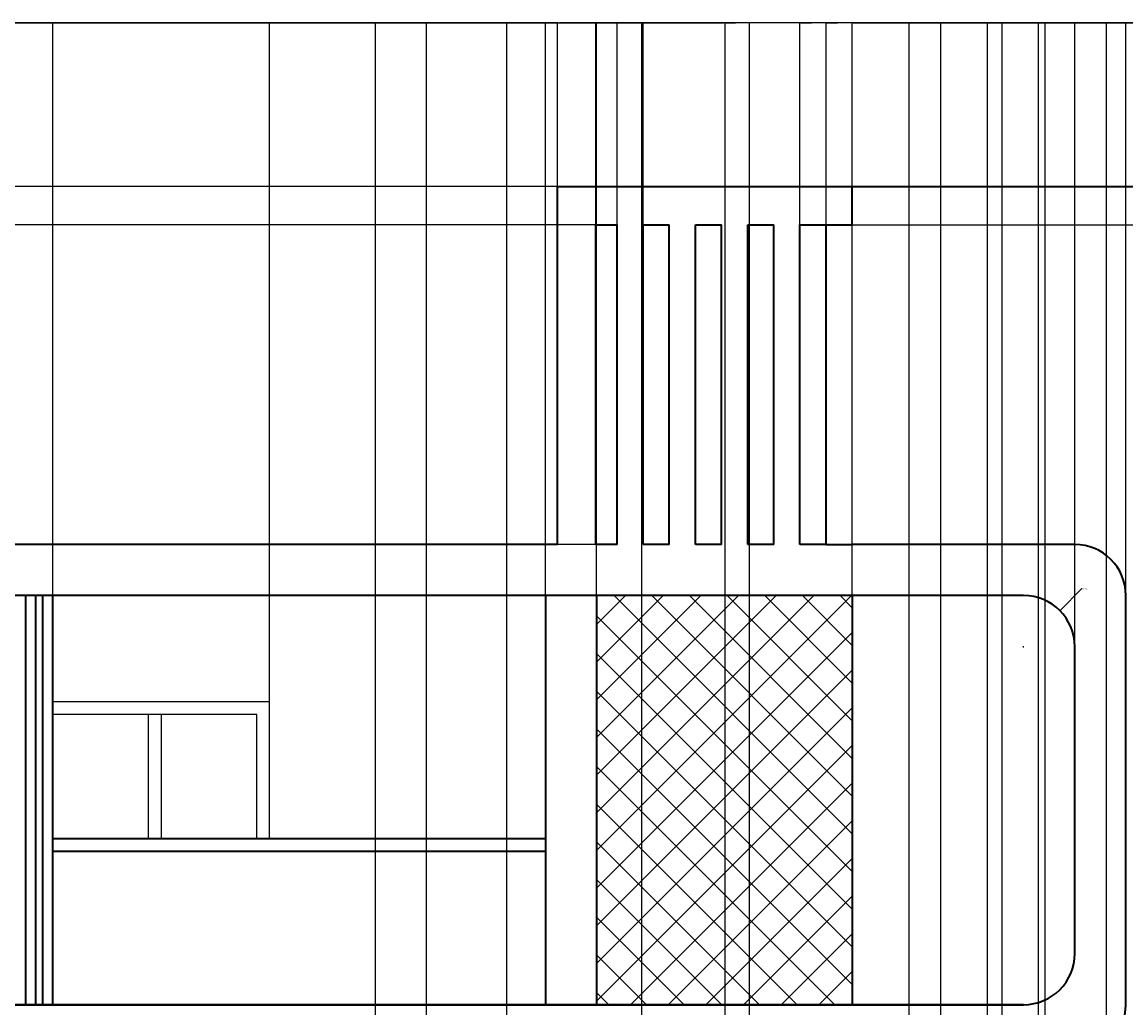
# Model space of a CAD drawing. Units: inches. Extents: x -15 to 605, y -220 to 570.
# Tile 9 of 10: x 138 to 397, y 339 to 570. Entities that reach past the tile are written whole.
import ezdxf

# ---------------------------------------------------------------- set-up
doc = ezdxf.new("R2010")
doc.units = ezdxf.units.IN
doc.header["$MEASUREMENT"] = 0
for name, color, linetype, lineweight in [('A-ANNO-DIMS', 2, 'Continuous', 18), ('A-ELEV', 7, 'Continuous', 35), ('A-ELEV-PATT', 8, 'Continuous', 13), ('A-GLAZ', 4, 'Continuous', 25)]:
    doc.layers.add(name, color=color, linetype=linetype, lineweight=lineweight)
doc.styles.get("Standard").update_dxf_attribs({"font": 'arial.ttf'})
doc.dimstyles.get("Standard").update_dxf_attribs({"dimtxt": 0.18, "dimasz": 0.18, "dimexe": 0.18, "dimexo": 0.0625, "dimgap": 0.09, "dimtad": 0, "dimtih": 1, "dimtoh": 1, "dimdec": 4, "dimzin": 0, "dimdsep": 46, "dimtxsty": 'Standard', "dimcen": 0.09, "dimadec": 0, "dimazin": 0, "dimtfac": 1, "dimtdec": 4, "dimtofl": 0, "dimtmove": 0, "dimatfit": 3, "dimfxl": 1, "dimtolj": 1, "dimtzin": 0, "dimarcsym": 0})

# ---------------------------------------------------------------- blocks, each defined once
blk = doc.blocks.new('WIN-ELEV')
for p, q in [((22.41, 29.07), (22.41, 0)), ((25.41, 29.07), (25.41, 0))]:
    blk.add_line(p, q)
for points in [[(50.87, 0), (50.87, 32.07), (0, 32.07)], [(47.87, 0), (47.87, 29.07), (0, 29.07)]]:
    blk.add_lwpolyline(points)
blk = doc.blocks.new('*D8')
at = {"layer": 'A-ANNO-DIMS', "color": 0, "lineweight": -2, "transparency": 16777216}
for p, q in [((23.99, 3.88), (23.99, 570.4)), ((24.17, 570.22), (263.7, 570.22)), ((503.81, 570.22), (264.28, 570.22)), ((503.99, 531.88), (503.99, 570.4))]:
    blk.add_line(p, q, dxfattribs=at)
at = {"layer": 'A-ANNO-DIMS', "color": 0, "transparency": 16777216}
for points in [[(24.17, 570.25), (24.17, 570.19), (23.99, 570.22)], [(503.81, 570.25), (503.81, 570.19), (503.99, 570.22)]]:
    blk.add_solid(points, dxfattribs=at)
at = {"layer": 'Defpoints', "color": 0, "transparency": 16777216}
for p in [(503.99, 570.22), (503.99, 531.82), (23.99, 3.82)]:
    blk.add_point(p, dxfattribs=at)
at = {"layer": 'A-ANNO-DIMS', "color": 0, "transparency": 16777216, "insert": (263.99, 570.22), "char_height": 0.18, "attachment_point": 5}
blk.add_mtext('\\A1;480', dxfattribs=at)
blk = doc.blocks.new('*D9')
at = {"layer": 'A-ANNO-DIMS', "color": 0, "lineweight": -2, "transparency": 16777216}
for p, q in [((503.92, 531.82), (-14.59, 531.82)), ((-14.41, 531.64), (-14.41, 208)), ((-14.41, -116), (-14.41, 207.64)), ((23.92, -116.18), (-14.59, -116.18))]:
    blk.add_line(p, q, dxfattribs=at)
at = {"layer": 'A-ANNO-DIMS', "color": 0, "transparency": 16777216}
for points in [[(-14.44, 531.64), (-14.38, 531.64), (-14.41, 531.82)], [(-14.44, -116), (-14.38, -116), (-14.41, -116.18)]]:
    blk.add_solid(points, dxfattribs=at)
at = {"layer": 'Defpoints', "color": 0, "transparency": 16777216}
for p in [(-14.41, 531.82), (503.99, 531.82), (23.99, -116.18)]:
    blk.add_point(p, dxfattribs=at)
at = {"layer": 'A-ANNO-DIMS', "color": 0, "transparency": 16777216, "insert": (-14.41, 207.82), "char_height": 0.18, "attachment_point": 5}
blk.add_mtext('\\A1;648', dxfattribs=at)
blk = doc.blocks.new('*D18')
at = {"layer": 'A-ANNO-DIMS', "color": 0, "lineweight": -2, "transparency": 16777216}
for p, q in [((23.99, 3.88), (23.99, 570.4)), ((24.17, 570.22), (143.44, 570.22)), ((263.64, 570.22), (144.37, 570.22)), ((263.82, 447.88), (263.82, 570.4))]:
    blk.add_line(p, q, dxfattribs=at)
at = {"layer": 'A-ANNO-DIMS', "color": 0, "transparency": 16777216}
for points in [[(24.17, 570.25), (24.17, 570.19), (23.99, 570.22)], [(263.64, 570.25), (263.64, 570.19), (263.82, 570.22)]]:
    blk.add_solid(points, dxfattribs=at)
at = {"layer": 'Defpoints', "color": 0, "transparency": 16777216}
for p in [(263.82, 570.22), (263.82, 447.82), (23.99, 3.82)]:
    blk.add_point(p, dxfattribs=at)
at = {"layer": 'A-ANNO-DIMS', "color": 0, "transparency": 16777216, "insert": (143.9, 570.22), "char_height": 0.18, "attachment_point": 5}
blk.add_mtext('\\A1;239.83', dxfattribs=at)
blk = doc.blocks.new('*D19')
at = {"layer": 'A-ANNO-DIMS', "color": 0, "lineweight": -2, "transparency": 16777216}
for p, q in [((263.82, 531.88), (263.82, 570.4)), ((264, 570.22), (298.01, 570.22)), ((332.81, 570.22), (298.8, 570.22)), ((332.99, 435.88), (332.99, 570.4))]:
    blk.add_line(p, q, dxfattribs=at)
at = {"layer": 'A-ANNO-DIMS', "color": 0, "transparency": 16777216}
for points in [[(264, 570.25), (264, 570.19), (263.82, 570.22)], [(332.81, 570.25), (332.81, 570.19), (332.99, 570.22)]]:
    blk.add_solid(points, dxfattribs=at)
at = {"layer": 'Defpoints', "color": 0, "transparency": 16777216}
for p in [(332.99, 570.22), (263.82, 531.82), (332.99, 435.82)]:
    blk.add_point(p, dxfattribs=at)
at = {"layer": 'A-ANNO-DIMS', "color": 0, "transparency": 16777216, "insert": (298.4, 570.22), "char_height": 0.18, "attachment_point": 5}
blk.add_mtext('\\A1;69.17', dxfattribs=at)
blk = doc.blocks.new('*D20')
at = {"layer": 'A-ANNO-DIMS', "color": 0, "lineweight": -2, "transparency": 16777216}
for p, q in [((332.99, 435.88), (332.99, 570.4)), ((333.17, 570.22), (418.22, 570.22)), ((503.81, 570.22), (418.75, 570.22)), ((503.99, 531.88), (503.99, 570.4))]:
    blk.add_line(p, q, dxfattribs=at)
at = {"layer": 'A-ANNO-DIMS', "color": 0, "transparency": 16777216}
for points in [[(333.17, 570.25), (333.17, 570.19), (332.99, 570.22)], [(503.81, 570.25), (503.81, 570.19), (503.99, 570.22)]]:
    blk.add_solid(points, dxfattribs=at)
at = {"layer": 'Defpoints', "color": 0, "transparency": 16777216}
for p in [(503.99, 570.22), (503.99, 531.82), (332.99, 435.82)]:
    blk.add_point(p, dxfattribs=at)
at = {"layer": 'A-ANNO-DIMS', "color": 0, "transparency": 16777216, "insert": (418.49, 570.22), "char_height": 0.18, "attachment_point": 5}
blk.add_mtext('\\A1;171', dxfattribs=at)
blk = doc.blocks.new('*D54')
at = {"layer": 'A-ANNO-DIMS', "color": 0, "lineweight": -2, "transparency": 16777216}
for p, q in [((63.91, -32.12), (63.91, 570.4)), ((64.09, 570.22), (142.07, 570.22)), ((220.96, 570.22), (142.98, 570.22)), ((221.14, -31.58), (221.14, 570.4))]:
    blk.add_line(p, q, dxfattribs=at)
at = {"layer": 'A-ANNO-DIMS', "color": 0, "transparency": 16777216}
for points in [[(64.09, 570.25), (64.09, 570.19), (63.91, 570.22)], [(220.96, 570.25), (220.96, 570.19), (221.14, 570.22)]]:
    blk.add_solid(points, dxfattribs=at)
at = {"layer": 'Defpoints', "color": 0, "transparency": 16777216}
for p in [(221.14, 570.22), (63.91, -32.18), (221.14, -31.64)]:
    blk.add_point(p, dxfattribs=at)
at = {"layer": 'A-ANNO-DIMS', "color": 0, "transparency": 16777216, "insert": (142.53, 570.22), "char_height": 0.18, "attachment_point": 5}
blk.add_mtext('\\A1;157.24', dxfattribs=at)
blk = doc.blocks.new('*D55')
at = {"layer": 'A-ANNO-DIMS', "color": 0, "lineweight": -2, "transparency": 16777216}
for p, q in [((221.14, -31.58), (221.14, 570.4)), ((221.32, 570.22), (226.93, 570.22)), ((232.96, 570.22), (227.35, 570.22)), ((233.14, -31.58), (233.14, 570.4))]:
    blk.add_line(p, q, dxfattribs=at)
at = {"layer": 'A-ANNO-DIMS', "color": 0, "transparency": 16777216}
for points in [[(221.32, 570.25), (221.32, 570.19), (221.14, 570.22)], [(232.96, 570.25), (232.96, 570.19), (233.14, 570.22)]]:
    blk.add_solid(points, dxfattribs=at)
at = {"layer": 'Defpoints', "color": 0, "transparency": 16777216}
for p in [(233.14, 570.22), (221.14, -31.64), (233.14, -31.64)]:
    blk.add_point(p, dxfattribs=at)
at = {"layer": 'A-ANNO-DIMS', "color": 0, "transparency": 16777216, "insert": (227.14, 570.22), "char_height": 0.18, "attachment_point": 5}
blk.add_mtext('\\A1;12', dxfattribs=at)
blk = doc.blocks.new('*D56')
at = {"layer": 'A-ANNO-DIMS', "color": 0, "lineweight": -2, "transparency": 16777216}
for p, q in [((233.14, -31.58), (233.14, 570.4)), ((233.32, 570.22), (298.47, 570.22)), ((364.53, 570.22), (299.38, 570.22)), ((364.71, -56.12), (364.71, 570.4))]:
    blk.add_line(p, q, dxfattribs=at)
at = {"layer": 'A-ANNO-DIMS', "color": 0, "transparency": 16777216}
for points in [[(233.32, 570.25), (233.32, 570.19), (233.14, 570.22)], [(364.53, 570.25), (364.53, 570.19), (364.71, 570.22)]]:
    blk.add_solid(points, dxfattribs=at)
at = {"layer": 'Defpoints', "color": 0, "transparency": 16777216}
for p in [(364.71, 570.22), (233.14, -31.64), (364.71, -56.18)]:
    blk.add_point(p, dxfattribs=at)
at = {"layer": 'A-ANNO-DIMS', "color": 0, "transparency": 16777216, "insert": (298.93, 570.22), "char_height": 0.18, "attachment_point": 5}
blk.add_mtext('\\A1;131.56', dxfattribs=at)
blk = doc.blocks.new('*D57')
at = {"layer": 'A-ANNO-DIMS', "color": 0, "lineweight": -2, "transparency": 16777216}
for p, q in [((364.71, -56.12), (364.71, 570.4)), ((364.89, 570.22), (370.5, 570.22)), ((376.53, 570.22), (370.92, 570.22)), ((376.71, -44.82), (376.71, 570.4))]:
    blk.add_line(p, q, dxfattribs=at)
at = {"layer": 'A-ANNO-DIMS', "color": 0, "transparency": 16777216}
for points in [[(364.89, 570.25), (364.89, 570.19), (364.71, 570.22)], [(376.53, 570.25), (376.53, 570.19), (376.71, 570.22)]]:
    blk.add_solid(points, dxfattribs=at)
at = {"layer": 'Defpoints', "color": 0, "transparency": 16777216}
for p in [(376.71, 570.22), (376.71, -44.88), (364.71, -56.18)]:
    blk.add_point(p, dxfattribs=at)
at = {"layer": 'A-ANNO-DIMS', "color": 0, "transparency": 16777216, "insert": (370.71, 570.22), "char_height": 0.18, "attachment_point": 5}
blk.add_mtext('\\A1;12', dxfattribs=at)
blk = doc.blocks.new('*D58')
at = {"layer": 'A-ANNO-DIMS', "color": 0, "lineweight": -2, "transparency": 16777216}
for p, q in [((376.71, -44.82), (376.71, 570.4)), ((376.89, 570.22), (419.58, 570.22)), ((462.92, 570.22), (420.23, 570.22)), ((463.1, -45.87), (463.1, 570.4))]:
    blk.add_line(p, q, dxfattribs=at)
at = {"layer": 'A-ANNO-DIMS', "color": 0, "transparency": 16777216}
for points in [[(376.89, 570.25), (376.89, 570.19), (376.71, 570.22)], [(462.92, 570.25), (462.92, 570.19), (463.1, 570.22)]]:
    blk.add_solid(points, dxfattribs=at)
at = {"layer": 'Defpoints', "color": 0, "transparency": 16777216}
for p in [(463.1, 570.22), (376.71, -44.88), (463.1, -45.94)]:
    blk.add_point(p, dxfattribs=at)
at = {"layer": 'A-ANNO-DIMS', "color": 0, "transparency": 16777216, "insert": (419.9, 570.22), "char_height": 0.18, "attachment_point": 5}
blk.add_mtext('\\A1;86.4', dxfattribs=at)
blk = doc.blocks.new('*D60')
at = {"layer": 'A-ANNO-DIMS', "color": 0, "lineweight": -2, "transparency": 16777216}
for p, q in [((346.37, -116.12), (346.37, 570.4)), ((346.55, 570.22), (349.67, 570.22)), ((353.57, 570.22), (350.45, 570.22)), ((353.75, -39.82), (353.75, 570.4))]:
    blk.add_line(p, q, dxfattribs=at)
at = {"layer": 'A-ANNO-DIMS', "color": 0, "transparency": 16777216}
for points in [[(346.55, 570.25), (346.55, 570.19), (346.37, 570.22)], [(353.57, 570.25), (353.57, 570.19), (353.75, 570.22)]]:
    blk.add_solid(points, dxfattribs=at)
at = {"layer": 'Defpoints', "color": 0, "transparency": 16777216}
for p in [(353.75, 570.22), (353.75, -39.88), (346.37, -116.18)]:
    blk.add_point(p, dxfattribs=at)
at = {"layer": 'A-ANNO-DIMS', "color": 0, "transparency": 16777216, "insert": (350.06, 570.22), "char_height": 0.18, "attachment_point": 5}
blk.add_mtext('\\A1;7.384', dxfattribs=at)
blk = doc.blocks.new('*D61')
at = {"layer": 'A-ANNO-DIMS', "color": 0, "lineweight": -2, "transparency": 16777216}
for p, q in [((353.75, -39.82), (353.75, 570.4)), ((353.93, 570.22), (360.55, 570.22)), ((367.95, 570.22), (361.33, 570.22)), ((368.13, -39.82), (368.13, 570.4))]:
    blk.add_line(p, q, dxfattribs=at)
at = {"layer": 'A-ANNO-DIMS', "color": 0, "transparency": 16777216}
for points in [[(353.93, 570.25), (353.93, 570.19), (353.75, 570.22)], [(367.95, 570.25), (367.95, 570.19), (368.13, 570.22)]]:
    blk.add_solid(points, dxfattribs=at)
at = {"layer": 'Defpoints', "color": 0, "transparency": 16777216}
for p in [(368.13, 570.22), (353.75, -39.88), (368.13, -39.88)]:
    blk.add_point(p, dxfattribs=at)
at = {"layer": 'A-ANNO-DIMS', "color": 0, "transparency": 16777216, "insert": (360.94, 570.22), "char_height": 0.18, "attachment_point": 5}
blk.add_mtext('\\A1;14.38', dxfattribs=at)
blk = doc.blocks.new('*D62')
at = {"layer": 'A-ANNO-DIMS', "color": 0, "lineweight": -2, "transparency": 16777216}
for p, q in [((378.23, -39.82), (378.23, 570.4)), ((378.41, 570.22), (385.04, 570.22)), ((392.43, 570.22), (385.81, 570.22)), ((392.61, -39.82), (392.61, 570.4))]:
    blk.add_line(p, q, dxfattribs=at)
at = {"layer": 'A-ANNO-DIMS', "color": 0, "transparency": 16777216}
for points in [[(378.41, 570.25), (378.41, 570.19), (378.23, 570.22)], [(392.43, 570.25), (392.43, 570.19), (392.61, 570.22)]]:
    blk.add_solid(points, dxfattribs=at)
at = {"layer": 'Defpoints', "color": 0, "transparency": 16777216}
for p in [(392.61, 570.22), (378.23, -39.88), (392.61, -39.88)]:
    blk.add_point(p, dxfattribs=at)
at = {"layer": 'A-ANNO-DIMS', "color": 0, "transparency": 16777216, "insert": (385.42, 570.22), "char_height": 0.18, "attachment_point": 5}
blk.add_mtext('\\A1;14.38', dxfattribs=at)
blk = doc.blocks.new('*D69')
at = {"layer": 'A-ANNO-DIMS', "color": 0, "lineweight": -2, "transparency": 16777216}
for p, q in [((263.82, 531.88), (263.82, 570.4)), ((264, 570.22), (268.17, 570.22)), ((272.64, 570.22), (268.47, 570.22)), ((272.82, 522.88), (272.82, 570.4))]:
    blk.add_line(p, q, dxfattribs=at)
at = {"layer": 'A-ANNO-DIMS', "color": 0, "transparency": 16777216}
for points in [[(264, 570.25), (264, 570.19), (263.82, 570.22)], [(272.64, 570.25), (272.64, 570.19), (272.82, 570.22)]]:
    blk.add_solid(points, dxfattribs=at)
at = {"layer": 'Defpoints', "color": 0, "transparency": 16777216}
for p in [(272.82, 570.22), (263.82, 531.82), (272.82, 522.82)]:
    blk.add_point(p, dxfattribs=at)
at = {"layer": 'A-ANNO-DIMS', "color": 0, "transparency": 16777216, "insert": (268.32, 570.22), "char_height": 0.18, "attachment_point": 5}
blk.add_mtext('\\A1;9', dxfattribs=at)
blk = doc.blocks.new('*D70')
at = {"layer": 'A-ANNO-DIMS', "color": 0, "lineweight": -2, "transparency": 16777216}
for p, q in [((272.82, 522.88), (272.82, 570.4)), ((273, 570.22), (274.91, 570.22)), ((277.62, 570.22), (275.71, 570.22)), ((277.8, 522.88), (277.8, 570.4))]:
    blk.add_line(p, q, dxfattribs=at)
at = {"layer": 'A-ANNO-DIMS', "color": 0, "transparency": 16777216}
for points in [[(273, 570.25), (273, 570.19), (272.82, 570.22)], [(277.62, 570.25), (277.62, 570.19), (277.8, 570.22)]]:
    blk.add_solid(points, dxfattribs=at)
at = {"layer": 'Defpoints', "color": 0, "transparency": 16777216}
for p in [(277.8, 570.22), (272.82, 522.82), (277.8, 522.82)]:
    blk.add_point(p, dxfattribs=at)
at = {"layer": 'A-ANNO-DIMS', "color": 0, "transparency": 16777216, "insert": (275.31, 570.22), "char_height": 0.18, "attachment_point": 5}
blk.add_mtext('\\A1;4.987', dxfattribs=at)
blk = doc.blocks.new('*D71')
at = {"layer": 'A-ANNO-DIMS', "color": 0, "lineweight": -2, "transparency": 16777216}
for p, q in [((277.8, 522.88), (277.8, 570.4)), ((277.98, 570.22), (280.48, 570.22)), ((283.75, 570.22), (281.26, 570.22)), ((283.93, 522.88), (283.93, 570.4))]:
    blk.add_line(p, q, dxfattribs=at)
at = {"layer": 'A-ANNO-DIMS', "color": 0, "transparency": 16777216}
for points in [[(277.98, 570.25), (277.98, 570.19), (277.8, 570.22)], [(283.75, 570.25), (283.75, 570.19), (283.93, 570.22)]]:
    blk.add_solid(points, dxfattribs=at)
at = {"layer": 'Defpoints', "color": 0, "transparency": 16777216}
for p in [(283.93, 570.22), (277.8, 522.82), (283.93, 522.82)]:
    blk.add_point(p, dxfattribs=at)
at = {"layer": 'A-ANNO-DIMS', "color": 0, "transparency": 16777216, "insert": (280.87, 570.22), "char_height": 0.18, "attachment_point": 5}
blk.add_mtext('\\A1;6.132', dxfattribs=at)
blk = doc.blocks.new('*D72')
at = {"layer": 'A-ANNO-DIMS', "color": 0, "lineweight": -2, "transparency": 16777216}
for p, q in [((320.72, 522.88), (320.72, 570.4)), ((320.9, 570.22), (323.4, 570.22)), ((326.68, 570.22), (324.18, 570.22)), ((326.86, 522.88), (326.86, 570.4))]:
    blk.add_line(p, q, dxfattribs=at)
at = {"layer": 'A-ANNO-DIMS', "color": 0, "transparency": 16777216}
for points in [[(320.9, 570.25), (320.9, 570.19), (320.72, 570.22)], [(326.68, 570.25), (326.68, 570.19), (326.86, 570.22)]]:
    blk.add_solid(points, dxfattribs=at)
at = {"layer": 'Defpoints', "color": 0, "transparency": 16777216}
for p in [(326.86, 570.22), (320.72, 522.82), (326.86, 522.82)]:
    blk.add_point(p, dxfattribs=at)
at = {"layer": 'A-ANNO-DIMS', "color": 0, "transparency": 16777216, "insert": (323.79, 570.22), "char_height": 0.18, "attachment_point": 5}
blk.add_mtext('\\A1;6.132', dxfattribs=at)
blk = doc.blocks.new('*D73')
at = {"layer": 'A-ANNO-DIMS', "color": 0, "lineweight": -2, "transparency": 16777216}
for p, q in [((326.86, 522.88), (326.86, 570.4)), ((327.04, 570.22), (329.53, 570.22)), ((332.81, 570.22), (330.31, 570.22)), ((332.99, 522.88), (332.99, 570.4))]:
    blk.add_line(p, q, dxfattribs=at)
at = {"layer": 'A-ANNO-DIMS', "color": 0, "transparency": 16777216}
for points in [[(327.04, 570.25), (327.04, 570.19), (326.86, 570.22)], [(332.81, 570.25), (332.81, 570.19), (332.99, 570.22)]]:
    blk.add_solid(points, dxfattribs=at)
at = {"layer": 'Defpoints', "color": 0, "transparency": 16777216}
for p in [(332.99, 570.22), (326.86, 522.82), (332.99, 522.82)]:
    blk.add_point(p, dxfattribs=at)
at = {"layer": 'A-ANNO-DIMS', "color": 0, "transparency": 16777216, "insert": (329.92, 570.22), "char_height": 0.18, "attachment_point": 5}
blk.add_mtext('\\A1;6.132', dxfattribs=at)
blk = doc.blocks.new('*D74')
at = {"layer": 'A-ANNO-DIMS', "color": 0, "lineweight": -2, "transparency": 16777216}
for p, q in [((272.75, 522.82), (-14.59, 522.82)), ((-14.41, 522.64), (-14.41, 485.5)), ((-14.41, 448), (-14.41, 485.14)), ((272.75, 447.82), (-14.59, 447.82))]:
    blk.add_line(p, q, dxfattribs=at)
at = {"layer": 'A-ANNO-DIMS', "color": 0, "transparency": 16777216}
for points in [[(-14.44, 522.64), (-14.38, 522.64), (-14.41, 522.82)], [(-14.44, 448), (-14.38, 448), (-14.41, 447.82)]]:
    blk.add_solid(points, dxfattribs=at)
at = {"layer": 'Defpoints', "color": 0, "transparency": 16777216}
for p in [(-14.41, 522.82), (272.82, 522.82), (272.82, 447.82)]:
    blk.add_point(p, dxfattribs=at)
at = {"layer": 'A-ANNO-DIMS', "color": 0, "transparency": 16777216, "insert": (-14.41, 485.32), "char_height": 0.18, "attachment_point": 5}
blk.add_mtext('\\A1;75', dxfattribs=at)
blk = doc.blocks.new('*D75')
at = {"layer": 'A-ANNO-DIMS', "color": 0, "lineweight": -2, "transparency": 16777216}
for p, q in [((333.05, 531.82), (605.3, 531.82)), ((605.12, 531.64), (605.12, 527.5)), ((605.12, 523), (605.12, 527.14)), ((333.05, 522.82), (605.3, 522.82))]:
    blk.add_line(p, q, dxfattribs=at)
at = {"layer": 'A-ANNO-DIMS', "color": 0, "transparency": 16777216}
for points in [[(605.09, 531.64), (605.15, 531.64), (605.12, 531.82)], [(605.09, 523), (605.15, 523), (605.12, 522.82)]]:
    blk.add_solid(points, dxfattribs=at)
at = {"layer": 'Defpoints', "color": 0, "transparency": 16777216}
for p in [(332.99, 531.82), (605.12, 531.82), (332.99, 522.82)]:
    blk.add_point(p, dxfattribs=at)
at = {"layer": 'A-ANNO-DIMS', "color": 0, "transparency": 16777216, "insert": (605.12, 527.32), "char_height": 0.18, "attachment_point": 5}
blk.add_mtext('\\A1;9', dxfattribs=at)
blk = doc.blocks.new('*D76')
at = {"layer": 'A-ANNO-DIMS', "color": 0, "lineweight": -2, "transparency": 16777216}
for p, q in [((272.92, 339.82), (-14.59, 339.82)), ((-14.41, 339.64), (-14.41, 334)), ((-14.41, 328), (-14.41, 333.64)), ((272.92, 327.82), (-14.59, 327.82))]:
    blk.add_line(p, q, dxfattribs=at)
at = {"layer": 'A-ANNO-DIMS', "color": 0, "transparency": 16777216}
for points in [[(-14.44, 339.64), (-14.38, 339.64), (-14.41, 339.82)], [(-14.44, 328), (-14.38, 328), (-14.41, 327.82)]]:
    blk.add_solid(points, dxfattribs=at)
at = {"layer": 'Defpoints', "color": 0, "transparency": 16777216}
for p in [(-14.41, 339.82), (272.99, 339.82), (272.99, 327.82)]:
    blk.add_point(p, dxfattribs=at)
at = {"layer": 'A-ANNO-DIMS', "color": 0, "transparency": 16777216, "insert": (-14.41, 333.82), "char_height": 0.18, "attachment_point": 5}
blk.add_mtext('\\A1;12', dxfattribs=at)
blk = doc.blocks.new('*D77')
at = {"layer": 'A-ANNO-DIMS', "color": 0, "lineweight": -2, "transparency": 16777216}
for p, q in [((272.92, 435.82), (-14.59, 435.82)), ((-14.41, 435.64), (-14.41, 388)), ((-14.41, 340), (-14.41, 387.64)), ((272.92, 339.82), (-14.59, 339.82))]:
    blk.add_line(p, q, dxfattribs=at)
at = {"layer": 'A-ANNO-DIMS', "color": 0, "transparency": 16777216}
for points in [[(-14.44, 435.64), (-14.38, 435.64), (-14.41, 435.82)], [(-14.44, 340), (-14.38, 340), (-14.41, 339.82)]]:
    blk.add_solid(points, dxfattribs=at)
at = {"layer": 'Defpoints', "color": 0, "transparency": 16777216}
for p in [(-14.41, 435.82), (272.99, 435.82), (272.99, 339.82)]:
    blk.add_point(p, dxfattribs=at)
at = {"layer": 'A-ANNO-DIMS', "color": 0, "transparency": 16777216, "insert": (-14.41, 387.82), "char_height": 0.18, "attachment_point": 5}
blk.add_mtext('\\A1;96', dxfattribs=at)
blk = doc.blocks.new('*D78')
at = {"layer": 'A-ANNO-DIMS', "color": 0, "lineweight": -2, "transparency": 16777216}
for p, q in [((272.75, 447.82), (-14.59, 447.82)), ((-14.41, 447.64), (-14.41, 442)), ((-14.41, 436), (-14.41, 441.64)), ((272.92, 435.82), (-14.59, 435.82))]:
    blk.add_line(p, q, dxfattribs=at)
at = {"layer": 'A-ANNO-DIMS', "color": 0, "transparency": 16777216}
for points in [[(-14.44, 447.64), (-14.38, 447.64), (-14.41, 447.82)], [(-14.44, 436), (-14.38, 436), (-14.41, 435.82)]]:
    blk.add_solid(points, dxfattribs=at)
at = {"layer": 'Defpoints', "color": 0, "transparency": 16777216}
for p in [(-14.41, 447.82), (272.82, 447.82), (272.99, 435.82)]:
    blk.add_point(p, dxfattribs=at)
at = {"layer": 'A-ANNO-DIMS', "color": 0, "transparency": 16777216, "insert": (-14.41, 441.82), "char_height": 0.18, "attachment_point": 5}
blk.add_mtext('\\A1;12', dxfattribs=at)
blk = doc.blocks.new('*D82')
at = {"layer": 'A-ANNO-DIMS', "color": 0, "lineweight": -2, "transparency": 16777216}
for p, q in [((123.03, 339.88), (123.03, 570.4)), ((123.21, 570.22), (133.9, 570.22)), ((145.25, 570.22), (134.55, 570.22)), ((145.43, 339.88), (145.43, 570.4))]:
    blk.add_line(p, q, dxfattribs=at)
at = {"layer": 'A-ANNO-DIMS', "color": 0, "transparency": 16777216}
for points in [[(123.21, 570.25), (123.21, 570.19), (123.03, 570.22)], [(145.25, 570.25), (145.25, 570.19), (145.43, 570.22)]]:
    blk.add_solid(points, dxfattribs=at)
at = {"layer": 'Defpoints', "color": 0, "transparency": 16777216}
for p in [(145.43, 570.22), (123.03, 339.82), (145.43, 339.82)]:
    blk.add_point(p, dxfattribs=at)
at = {"layer": 'A-ANNO-DIMS', "color": 0, "transparency": 16777216, "insert": (134.23, 570.22), "char_height": 0.18, "attachment_point": 5}
blk.add_mtext('\\A1;22.4', dxfattribs=at)
blk = doc.blocks.new('*D83')
at = {"layer": 'A-ANNO-DIMS', "color": 0, "lineweight": -2, "transparency": 16777216}
for p, q in [((145.43, 339.88), (145.43, 570.4)), ((145.61, 570.22), (170.47, 570.22)), ((196.11, 570.22), (171.25, 570.22)), ((196.29, 378.88), (196.29, 570.4))]:
    blk.add_line(p, q, dxfattribs=at)
at = {"layer": 'A-ANNO-DIMS', "color": 0, "transparency": 16777216}
for points in [[(145.61, 570.25), (145.61, 570.19), (145.43, 570.22)], [(196.11, 570.25), (196.11, 570.19), (196.29, 570.22)]]:
    blk.add_solid(points, dxfattribs=at)
at = {"layer": 'Defpoints', "color": 0, "transparency": 16777216}
for p in [(196.29, 570.22), (196.29, 378.82), (145.43, 339.82)]:
    blk.add_point(p, dxfattribs=at)
at = {"layer": 'A-ANNO-DIMS', "color": 0, "transparency": 16777216, "insert": (170.86, 570.22), "char_height": 0.18, "attachment_point": 5}
blk.add_mtext('\\A1;50.87', dxfattribs=at)
blk = doc.blocks.new('*D84')
at = {"layer": 'A-ANNO-DIMS', "color": 0, "lineweight": -2, "transparency": 16777216}
for p, q in [((196.29, 378.88), (196.29, 570.4)), ((196.47, 570.22), (228.25, 570.22)), ((260.81, 570.22), (229.04, 570.22)), ((260.99, 339.88), (260.99, 570.4))]:
    blk.add_line(p, q, dxfattribs=at)
at = {"layer": 'A-ANNO-DIMS', "color": 0, "transparency": 16777216}
for points in [[(196.47, 570.25), (196.47, 570.19), (196.29, 570.22)], [(260.81, 570.25), (260.81, 570.19), (260.99, 570.22)]]:
    blk.add_solid(points, dxfattribs=at)
at = {"layer": 'Defpoints', "color": 0, "transparency": 16777216}
for p in [(260.99, 570.22), (196.29, 378.82), (260.99, 339.82)]:
    blk.add_point(p, dxfattribs=at)
at = {"layer": 'A-ANNO-DIMS', "color": 0, "transparency": 16777216, "insert": (228.64, 570.22), "char_height": 0.18, "attachment_point": 5}
blk.add_mtext('\\A1;64.69', dxfattribs=at)
blk = doc.blocks.new('*D85')
at = {"layer": 'A-ANNO-DIMS', "color": 0, "lineweight": -2, "transparency": 16777216}
for p, q in [((260.99, 339.88), (260.99, 570.4)), ((261.17, 570.22), (266.78, 570.22)), ((272.81, 570.22), (267.2, 570.22)), ((272.99, 339.88), (272.99, 570.4))]:
    blk.add_line(p, q, dxfattribs=at)
at = {"layer": 'A-ANNO-DIMS', "color": 0, "transparency": 16777216}
for points in [[(261.17, 570.25), (261.17, 570.19), (260.99, 570.22)], [(272.81, 570.25), (272.81, 570.19), (272.99, 570.22)]]:
    blk.add_solid(points, dxfattribs=at)
at = {"layer": 'Defpoints', "color": 0, "transparency": 16777216}
for p in [(272.99, 570.22), (260.99, 339.82), (272.99, 339.82)]:
    blk.add_point(p, dxfattribs=at)
at = {"layer": 'A-ANNO-DIMS', "color": 0, "transparency": 16777216, "insert": (266.99, 570.22), "char_height": 0.18, "attachment_point": 5}
blk.add_mtext('\\A1;12', dxfattribs=at)
blk = doc.blocks.new('*D86')
at = {"layer": 'A-ANNO-DIMS', "color": 0, "lineweight": -2, "transparency": 16777216}
for p, q in [((272.99, 339.88), (272.99, 570.4)), ((273.17, 570.22), (302.77, 570.22)), ((332.81, 570.22), (303.21, 570.22)), ((332.99, 339.88), (332.99, 570.4))]:
    blk.add_line(p, q, dxfattribs=at)
at = {"layer": 'A-ANNO-DIMS', "color": 0, "transparency": 16777216}
for points in [[(273.17, 570.25), (273.17, 570.19), (272.99, 570.22)], [(332.81, 570.25), (332.81, 570.19), (332.99, 570.22)]]:
    blk.add_solid(points, dxfattribs=at)
at = {"layer": 'Defpoints', "color": 0, "transparency": 16777216}
for p in [(332.99, 570.22), (272.99, 339.82), (332.99, 339.82)]:
    blk.add_point(p, dxfattribs=at)
at = {"layer": 'A-ANNO-DIMS', "color": 0, "transparency": 16777216, "insert": (302.99, 570.22), "char_height": 0.18, "attachment_point": 5}
blk.add_mtext('\\A1;60', dxfattribs=at)
blk = doc.blocks.new('*D87')
at = {"layer": 'A-ANNO-DIMS', "color": 0, "lineweight": -2, "transparency": 16777216}
for p, q in [((332.99, 339.88), (332.99, 570.4)), ((333.17, 570.22), (358.77, 570.22)), ((385.01, 570.22), (359.41, 570.22)), ((385.19, 351.88), (385.19, 570.4))]:
    blk.add_line(p, q, dxfattribs=at)
at = {"layer": 'A-ANNO-DIMS', "color": 0, "transparency": 16777216}
for points in [[(333.17, 570.25), (333.17, 570.19), (332.99, 570.22)], [(385.01, 570.25), (385.01, 570.19), (385.19, 570.22)]]:
    blk.add_solid(points, dxfattribs=at)
at = {"layer": 'Defpoints', "color": 0, "transparency": 16777216}
for p in [(385.19, 570.22), (385.19, 351.82), (332.99, 339.82)]:
    blk.add_point(p, dxfattribs=at)
at = {"layer": 'A-ANNO-DIMS', "color": 0, "transparency": 16777216, "insert": (359.09, 570.22), "char_height": 0.18, "attachment_point": 5}
blk.add_mtext('\\A1;52.2', dxfattribs=at)
blk = doc.blocks.new('*D88')
at = {"layer": 'A-ANNO-DIMS', "color": 0, "lineweight": -2, "transparency": 16777216}
for p, q in [((385.19, 351.88), (385.19, 570.4)), ((385.37, 570.22), (390.98, 570.22)), ((397.01, 570.22), (391.4, 570.22)), ((397.19, 339.88), (397.19, 570.4))]:
    blk.add_line(p, q, dxfattribs=at)
at = {"layer": 'A-ANNO-DIMS', "color": 0, "transparency": 16777216}
for points in [[(385.37, 570.25), (385.37, 570.19), (385.19, 570.22)], [(397.01, 570.25), (397.01, 570.19), (397.19, 570.22)]]:
    blk.add_solid(points, dxfattribs=at)
at = {"layer": 'Defpoints', "color": 0, "transparency": 16777216}
for p in [(397.19, 570.22), (385.19, 351.82), (397.19, 339.82)]:
    blk.add_point(p, dxfattribs=at)
at = {"layer": 'A-ANNO-DIMS', "color": 0, "transparency": 16777216, "insert": (391.19, 570.22), "char_height": 0.18, "attachment_point": 5}
blk.add_mtext('\\A1;12', dxfattribs=at)
blk = doc.blocks.new('*D104')
at = {"layer": 'A-ANNO-DIMS', "color": 0, "lineweight": -2, "transparency": 16777216}
for p, q in [((251.99, -56.12), (251.99, 570.4)), ((252.17, 570.22), (267.39, 570.22)), ((283.41, 570.22), (268.18, 570.22)), ((283.59, -84.79), (283.59, 570.4))]:
    blk.add_line(p, q, dxfattribs=at)
at = {"layer": 'A-ANNO-DIMS', "color": 0, "transparency": 16777216}
for points in [[(252.17, 570.25), (252.17, 570.19), (251.99, 570.22)], [(283.41, 570.25), (283.41, 570.19), (283.59, 570.22)]]:
    blk.add_solid(points, dxfattribs=at)
at = {"layer": 'Defpoints', "color": 0, "transparency": 16777216}
for p in [(283.59, 570.22), (251.99, -56.18), (283.59, -84.86)]:
    blk.add_point(p, dxfattribs=at)
at = {"layer": 'A-ANNO-DIMS', "color": 0, "transparency": 16777216, "insert": (267.79, 570.22), "char_height": 0.18, "attachment_point": 5}
blk.add_mtext('\\A1;31.60', dxfattribs=at)
blk = doc.blocks.new('*D105')
at = {"layer": 'A-ANNO-DIMS', "color": 0, "lineweight": -2, "transparency": 16777216}
for p, q in [((283.59, -84.79), (283.59, 570.4)), ((283.77, 570.22), (292.92, 570.22)), ((302.99, 570.22), (293.84, 570.22)), ((303.17, -103.62), (303.17, 570.4))]:
    blk.add_line(p, q, dxfattribs=at)
at = {"layer": 'A-ANNO-DIMS', "color": 0, "transparency": 16777216}
for points in [[(283.77, 570.25), (283.77, 570.19), (283.59, 570.22)], [(302.99, 570.25), (302.99, 570.19), (303.17, 570.22)]]:
    blk.add_solid(points, dxfattribs=at)
at = {"layer": 'Defpoints', "color": 0, "transparency": 16777216}
for p in [(303.17, 570.22), (283.59, -84.86), (303.17, -103.68)]:
    blk.add_point(p, dxfattribs=at)
at = {"layer": 'A-ANNO-DIMS', "color": 0, "transparency": 16777216, "insert": (293.38, 570.22), "char_height": 0.18, "attachment_point": 5}
blk.add_mtext('\\A1;19.585', dxfattribs=at)
blk = doc.blocks.new('*D106')
at = {"layer": 'A-ANNO-DIMS', "color": 0, "lineweight": -2, "transparency": 16777216}
for p, q in [((303.17, -103.62), (303.17, 570.4)), ((303.35, 570.22), (305.62, 570.22)), ((308.68, 570.22), (306.41, 570.22)), ((308.86, -79.16), (308.86, 570.4))]:
    blk.add_line(p, q, dxfattribs=at)
at = {"layer": 'A-ANNO-DIMS', "color": 0, "transparency": 16777216}
for points in [[(303.35, 570.25), (303.35, 570.19), (303.17, 570.22)], [(308.68, 570.25), (308.68, 570.19), (308.86, 570.22)]]:
    blk.add_solid(points, dxfattribs=at)
at = {"layer": 'Defpoints', "color": 0, "transparency": 16777216}
for p in [(308.86, 570.22), (308.86, -79.22), (303.17, -103.68)]:
    blk.add_point(p, dxfattribs=at)
at = {"layer": 'A-ANNO-DIMS', "color": 0, "transparency": 16777216, "insert": (306.02, 570.22), "char_height": 0.18, "attachment_point": 5}
blk.add_mtext('\\A1;5.689', dxfattribs=at)
blk = doc.blocks.new('*D122')
at = {"layer": 'A-ANNO-DIMS', "color": 0, "lineweight": -2, "transparency": 16777216}
for p, q in [((386.77, 437.39), (381.81, 432.43)), ((386.95, 437.39), (386.77, 437.39)), ((373.1, 423.82), (373.28, 423.82)), ((373.19, 423.73), (373.19, 423.91))]:
    blk.add_line(p, q, dxfattribs=at)
at = {"layer": 'A-ANNO-DIMS', "color": 0, "transparency": 16777216}
blk.add_solid([(381.79, 432.45), (381.83, 432.41), (381.68, 432.3)], dxfattribs=at)
at = {"layer": 'Defpoints', "color": 0, "transparency": 16777216}
for p in [(381.68, 432.3), (373.19, 423.82)]:
    blk.add_point(p, dxfattribs=at)
at = {"layer": 'A-ANNO-DIMS', "color": 0, "transparency": 16777216, "insert": (387.63, 437.39), "char_height": 0.18, "attachment_point": 5}
blk.add_mtext('\\A1;4X R12.00', dxfattribs=at)

msp = doc.modelspace()

# ---------------------------------------------------------------- hatches: boundary and pattern name
at = {"layer": 'A-ELEV-PATT'}
h = msp.add_hatch(dxfattribs=at)
h.set_pattern_fill('ANSI37', color=256, scale=50)
h.set_pattern_definition([(45, (0, 324), (-4.41942, 4.41942), []), (135, (0, 324), (-4.41942, -4.41942), [])])
h.paths.add_polyline_path([(332.9872, 435.8187), (272.9872, 435.8187), (272.9872, 339.8187), (332.9872, 339.8187)])

# ---------------------------------------------------------------- linework, layer by layer
at = {"layer": 'A-ELEV'}
for p, q in [((263.8163, 531.8187), (503.9872, 531.8187)), ((263.8163, 447.8187), (263.8163, 531.8187)), ((332.9872, 522.8187), (332.9872, 531.8187)), ((272.8163, 447.8187), (272.8163, 522.8187)), ((272.8163, 522.8187), (277.8031, 522.8187)), ((277.8031, 447.8187), (277.8031, 522.8187)), ((283.9346, 447.8187), (283.9346, 522.8187)), ((283.9346, 522.8187), (290.0662, 522.8187)), ((290.0662, 447.8187), (290.0662, 522.8187)), ((296.1978, 447.8187), (296.1978, 522.8187)), ((296.1978, 522.8187), (302.3294, 522.8187)), ((302.3294, 447.8187), (302.3294, 522.8187)), ((308.4609, 447.8187), (308.4609, 522.8187)), ((308.4609, 522.8187), (314.5925, 522.8187)), ((314.5925, 447.8187), (314.5925, 522.8187)), ((320.7241, 447.8187), (320.7241, 522.8187)), ((320.7241, 522.8187), (326.8557, 522.8187)), ((326.8557, 447.8187), (326.8557, 522.8187)), ((326.8557, 522.8187), (332.9872, 522.8187)), ((263.8163, 447.8187), (32.9872, 447.8187)), ((277.8031, 447.8187), (272.8163, 447.8187)), ((277.8031, 447.8187), (272.8163, 447.8187)), ((290.0662, 447.8187), (283.9346, 447.8187)), ((290.0662, 447.8187), (283.9346, 447.8187)), ((302.3294, 447.8187), (296.1978, 447.8187)), ((302.3294, 447.8187), (296.1978, 447.8187)), ((314.5925, 447.8187), (308.4609, 447.8187)), ((314.5925, 447.8187), (308.4609, 447.8187)), ((326.8557, 447.8187), (320.7241, 447.8187)), ((326.8557, 447.8187), (320.7241, 447.8187)), ((326.8557, 447.8187), (332.9872, 447.8187)), ((385.1921, 447.8187), (332.9872, 447.8187)), ((385.1921, 447.8187), (332.9872, 447.8187)), ((373.1921, 435.8187), (44.9872, 435.8187)), ((260.9872, 435.8187), (260.9872, 339.8187)), ((272.9872, 435.8187), (272.9872, 339.8187)), ((332.9872, 435.8187), (332.9872, 339.8187)), ((397.1921, 339.8187), (397.1921, 435.8187)), ((385.1921, 351.8187), (385.1921, 423.8187)), ((373.1921, 339.8187), (44.9872, 339.8187)), ((54.933, 339.8187), (212.3003, 339.8187)), ((212.3003, 339.8187), (260.9872, 339.8187)), ((260.9872, 339.8187), (373.1921, 339.8187))]:
    msp.add_line(p, q, dxfattribs=at)
for points in [[(139.027, 435.8187), (139.027, 339.8187), (141.4271, 339.8187), (141.4271, 435.8187)], [(143.0272, 435.8187), (143.0272, 339.8187), (145.4272, 339.8187), (145.4272, 435.8187)], [(145.4272, 378.8187), (212.3003, 378.8187), (260.9872, 378.8187)], [(145.4272, 375.8187), (212.3003, 375.8187), (260.9872, 375.8187)]]:
    msp.add_lwpolyline(points, dxfattribs=at)
for centre, start, end in [((385.1921, 435.8187), 0, 90), ((373.1921, 423.8187), 0, 90), ((373.1921, 351.8187), 270, 0), ((385.1921, 339.8187), 270, 0)]:
    msp.add_arc(centre, 12, start, end, dxfattribs=at)

# ---------------------------------------------------------------- block references
at = {"layer": 'A-GLAZ'}
msp.add_blockref('WIN-ELEV', (145.427, 378.819), dxfattribs=at)

# ---------------------------------------------------------------- dimensions: what is measured, and where the dimension line sits
at = {"layer": 'A-ANNO-DIMS'}
for base, p1, p2, override, picture, middle in [((503.9872, 570.2187), (23.9872, 3.8187), (503.9872, 531.8187), {"dimdec": 0, "dimlfac": 1, "dimrnd": 0, "dimzin": 0, "dimdsep": 46, "dimlunit": 2}, '*D8', (263.9872, 570.2187)), ((263.8163, 570.2187), (23.9872, 3.8187), (263.8163, 447.8187), {"dimdec": 2, "dimlfac": 1, "dimrnd": 0, "dimzin": 0, "dimdsep": 46, "dimlunit": 2}, '*D18', (143.9018, 570.2187)), ((221.1439, 570.2187), (63.9067, -32.1813), (221.1439, -31.6396), {"dimdec": 2, "dimlfac": 1, "dimrnd": 0, "dimzin": 0, "dimdsep": 46, "dimlunit": 2}, '*D54', (142.5253, 570.2187)), ((145.4272, 570.2187), (123.0266, 339.8187), (145.4272, 339.8187), {"dimdec": 1, "dimlfac": 1, "dimrnd": 0, "dimzin": 0, "dimdsep": 46, "dimlunit": 2}, '*D82', (134.2269, 570.2187)), ((196.294, 570.2187), (145.4272, 339.8187), (196.294, 378.8187), {"dimdec": 2, "dimlfac": 1, "dimrnd": 0, "dimzin": 0, "dimdsep": 46, "dimlunit": 2}, '*D83', (170.8606, 570.2187)), ((260.9872, 570.2187), (196.294, 378.8187), (260.9872, 339.8187), {"dimdec": 2, "dimlfac": 1, "dimrnd": 0, "dimzin": 0, "dimdsep": 46, "dimlunit": 2}, '*D84', (228.6406, 570.2187)), ((233.1439, 570.2187), (221.1439, -31.6396), (233.1439, -31.6396), {"dimdec": 0, "dimlfac": 1, "dimrnd": 0, "dimzin": 0, "dimdsep": 46, "dimlunit": 2}, '*D55', (227.1439, 570.2187)), ((364.7066, 570.2187), (233.1439, -31.6396), (364.7066, -56.1813), {"dimdec": 2, "dimlfac": 1, "dimrnd": 0, "dimzin": 0, "dimdsep": 46, "dimlunit": 2}, '*D56', (298.9252, 570.2187)), ((283.5871, 570.2187), (251.9872, -56.1813), (283.5871, -84.8572), {"dimdec": 2, "dimlfac": 1, "dimrnd": 0, "dimzin": 0, "dimdsep": 46, "dimlunit": 2}, '*D104', (267.7872, 570.2187)), ((272.9872, 570.2187), (260.9872, 339.8187), (272.9872, 339.8187), {"dimdec": 0, "dimlfac": 1, "dimrnd": 0, "dimzin": 0, "dimdsep": 46, "dimlunit": 2}, '*D85', (266.9872, 570.2187)), ((332.9872, 570.2187), (263.8163, 531.8187), (332.9872, 435.8187), {"dimdec": 2, "dimlfac": 1, "dimrnd": 0, "dimzin": 0, "dimdsep": 46, "dimlunit": 2}, '*D19', (298.4018, 570.2187)), ((272.8163, 570.2187), (263.8163, 531.8187), (272.8163, 522.8187), {"dimdec": 0, "dimlfac": 1, "dimrnd": 0, "dimzin": 0, "dimdsep": 46, "dimlunit": 2}, '*D69', (268.3163, 570.2187)), ((277.8031, 570.2187), (272.8163, 522.8187), (277.8031, 522.8187), {"dimdec": 3, "dimlfac": 1, "dimrnd": 0, "dimzin": 0, "dimdsep": 46, "dimlunit": 2}, '*D70', (275.3097, 570.2187)), ((332.9872, 570.2187), (272.9872, 339.8187), (332.9872, 339.8187), {"dimdec": 0, "dimlfac": 1, "dimrnd": 0, "dimzin": 0, "dimdsep": 46, "dimlunit": 2}, '*D86', (302.9872, 570.2187)), ((283.93464, 570.21873), (277.80307, 522.81873), (283.93464, 522.81873), {"dimdec": 3, "dimlfac": 1, "dimrnd": 0, "dimzin": 0, "dimdsep": 46, "dimlunit": 2}, '*D71', (280.86885, 570.21873)), ((303.1719, 570.2187), (283.5871, -84.8572), (303.1719, -103.6786), {"dimdec": 3, "dimlfac": 1, "dimrnd": 0, "dimzin": 0, "dimdsep": 46, "dimlunit": 2}, '*D105', (293.3795, 570.2187)), ((308.8611, 570.2187), (303.1719, -103.6786), (308.8611, -79.2202), {"dimdec": 3, "dimlfac": 1, "dimrnd": 0, "dimzin": 0, "dimdsep": 46, "dimlunit": 2}, '*D106', (306.0165, 570.2187)), ((326.8557, 570.2187), (320.7241, 522.8187), (326.8557, 522.8187), {"dimdec": 3, "dimlfac": 1, "dimrnd": 0, "dimzin": 0, "dimdsep": 46, "dimlunit": 2}, '*D72', (323.7899, 570.2187)), ((332.98723, 570.21873), (326.85566, 522.81873), (332.98723, 522.81873), {"dimdec": 3, "dimlfac": 1, "dimrnd": 0, "dimzin": 0, "dimdsep": 46, "dimlunit": 2}, '*D73', (329.92145, 570.21873)), ((503.9872, 570.2187), (332.9872, 435.8187), (503.9872, 531.8187), {"dimdec": 0, "dimlfac": 1, "dimrnd": 0, "dimzin": 0, "dimdsep": 46, "dimlunit": 2}, '*D20', (418.4872, 570.2187)), ((385.1921, 570.2187), (332.9872, 339.8187), (385.1921, 351.8187), {"dimdec": 1, "dimlfac": 1, "dimrnd": 0, "dimzin": 0, "dimdsep": 46, "dimlunit": 2}, '*D87', (359.0897, 570.2187)), ((353.7501, 570.2187), (346.3663, -116.1813), (353.7501, -39.8843), {"dimdec": 3, "dimlfac": 1, "dimrnd": 0, "dimzin": 0, "dimdsep": 46, "dimlunit": 2}, '*D60', (350.0582, 570.2187)), ((368.1292, 570.2187), (353.7501, -39.8843), (368.1292, -39.8843), {"dimdec": 2, "dimlfac": 1, "dimrnd": 0, "dimzin": 0, "dimdsep": 46, "dimlunit": 2}, '*D61', (360.9397, 570.2187)), ((376.7066, 570.2187), (364.7066, -56.1813), (376.7066, -44.8803), {"dimdec": 0, "dimlfac": 1, "dimrnd": 0, "dimzin": 0, "dimdsep": 46, "dimlunit": 2}, '*D57', (370.7066, 570.2187)), ((463.1032, 570.2187), (376.7066, -44.8803), (463.1032, -45.9373), {"dimdec": 1, "dimlfac": 1, "dimrnd": 0, "dimzin": 0, "dimdsep": 46, "dimlunit": 2}, '*D58', (419.9049, 570.2187)), ((392.6125, 570.2187), (378.2334, -39.8843), (392.6125, -39.8843), {"dimdec": 2, "dimlfac": 1, "dimrnd": 0, "dimzin": 0, "dimdsep": 46, "dimlunit": 2}, '*D62', (385.423, 570.2187)), ((397.1921, 570.2187), (385.1921, 351.8187), (397.1921, 339.8187), {"dimdec": 0, "dimlfac": 1, "dimrnd": 0, "dimzin": 0, "dimdsep": 46, "dimlunit": 2}, '*D88', (391.1921, 570.2187))]:
    dim = msp.add_linear_dim(base=base, p1=p1, p2=p2, dimstyle='Standard', override=override, dxfattribs=at)
    dim.commit()
    dim.dimension.update_dxf_attribs({"geometry": picture, "text_midpoint": middle})
for base, p1, p2, picture, middle in [((-14.4128, 531.8187), (23.9872, -116.1813), (503.9872, 531.8187), '*D9', (-14.4128, 207.8187)), ((605.1161, 531.8187), (332.9872, 522.8187), (332.9872, 531.8187), '*D75', (605.1161, 527.3187)), ((-14.4128, 522.8187), (272.8163, 447.8187), (272.8163, 522.8187), '*D74', (-14.4128, 485.3187)), ((-14.4128, 447.8187), (272.9872, 435.8187), (272.8163, 447.8187), '*D78', (-14.4128, 441.8187)), ((-14.4128, 435.8187), (272.9872, 339.8187), (272.9872, 435.8187), '*D77', (-14.4128, 387.8187)), ((-14.4128, 339.8187), (272.9872, 327.8187), (272.9872, 339.8187), '*D76', (-14.4128, 333.8187))]:
    dim = msp.add_linear_dim(base=base, p1=p1, p2=p2, angle=90, dimstyle='Standard', override={"dimdec": 0, "dimlfac": 1, "dimrnd": 0, "dimzin": 0, "dimdsep": 46, "dimlunit": 2}, dxfattribs=at)
    dim.commit()
    dim.dimension.update_dxf_attribs({"geometry": picture, "text_midpoint": middle})
dim = msp.add_radius_dim(center=(373.1921, 423.8187), mpoint=(381.6792, 432.3022), text='4X <>', dimstyle='Standard', override={"dimdec": 2, "dimlfac": 1, "dimrnd": 0, "dimzin": 0, "dimdsep": 46, "dimlunit": 2}, dxfattribs=at)
dim.commit()
dim.dimension.update_dxf_attribs({"geometry": '*D122', "text_midpoint": (387.628, 437.3923), "dimtype": 164})

doc.saveas('drawing.dxf')
